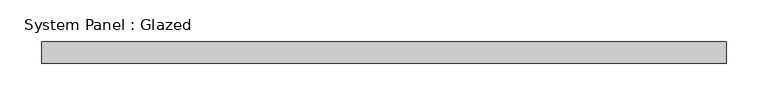
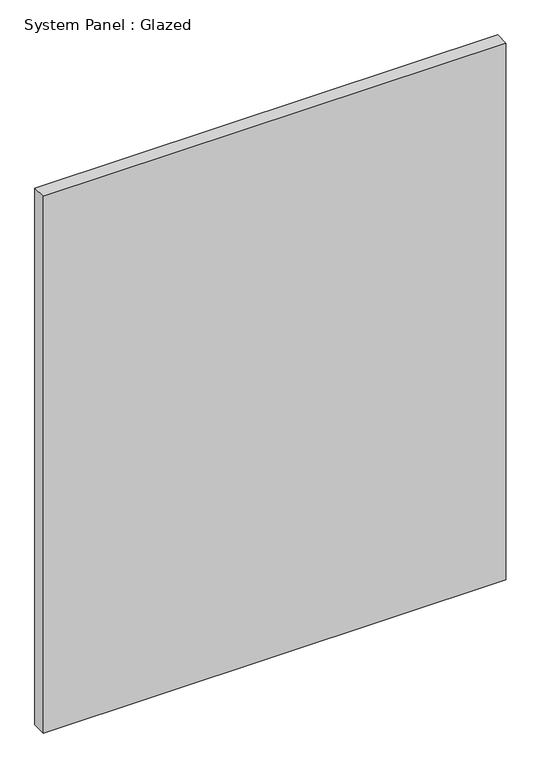
"""IFC4 building model written with IfcOpenShell, lengths in millimetres: plate geometry, System Panel : Glazed."""

from ifc_helpers import new_model, si_unit, origin, origin_with_axes, place, context, project, spatial, polyline, outline, extrude, source, transform, mapped, element, save


def system_panel_glazed_46c6fbea(model_context):
    return source(origin(), model_context, "Body", "SweptSolid", [
        extrude(outline(polyline([(409.5750001, 19.05), (-409.5750001, 19.05), (-409.5750001, 44.45), (409.5750001, 44.45), (409.5750001, 19.05)])), origin_with_axes(), (0.0, 0.0, 1.0), 1004.3270399),
    ])


if __name__ == "__main__":
    model = new_model("IFC4")
    model_context = context("Model", 3, world=origin())
    ifc_project = project(units=[si_unit("LENGTHUNIT", "METRE", prefix="MILLI")], contexts=[model_context])
    site = spatial("IfcSite", under=ifc_project)
    building = spatial("IfcBuilding", under=site)
    placement = place(None, origin())
    system_panel_glazed_shape = system_panel_glazed_46c6fbea(model_context)
    element("IfcPlate", 1, ObjectType="System Panel : Glazed", at=placement, inside=building, context=model_context, shape_type="MappedRepresentation", body=[
        mapped(system_panel_glazed_shape, transform((0.0, 0.0, 0.0), x_axis=(1.0, 0.0, 0.0), y_axis=(0.0, 1.0, 0.0), z_axis=(0.0, 0.0, 1.0))),
    ])
    save(model, "model.ifc")

# Revit data of these elements
# Type "System Panel : Glazed"
#   Construction Type Id = "GSP4R"
#   Analytic Construction = "1/8 in Pilkington single glazing"
#   Visual Light Transmittance = 0.9
#   Solar Heat Gain Coefficient = 0.86
#   Heat Transfer Coefficient (U) = 1.18115 BTU/(h·ft²·°F)
#   Define Thermal Properties by = 1
# Element 1 (IfcPlate, "System Panel : Glazed")
#   Materials on its faces: "Glass"
# Materials
#   "Glass": class "Glass", colour RGB 0 128 192, transparency 0.75, Description = "Soda Lime Glass", Cost = 0
